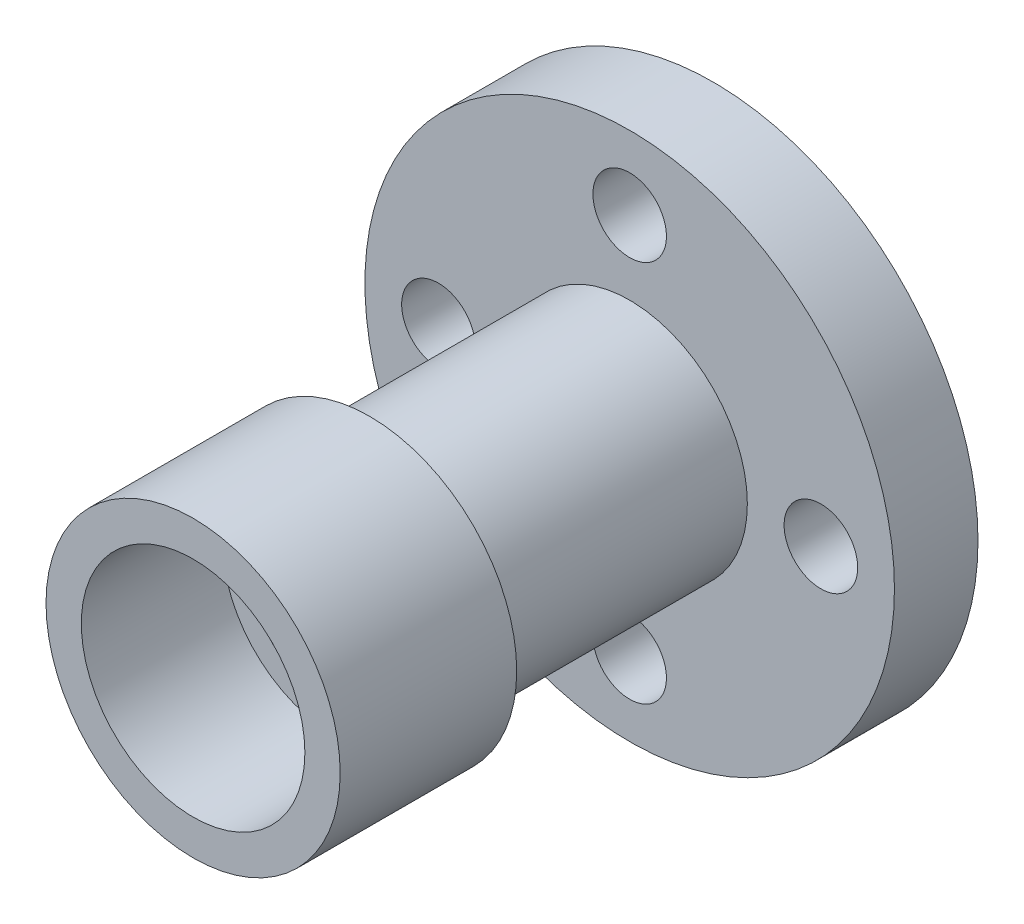
ISO-10303-21;
HEADER;
FILE_DESCRIPTION(('STEP AP214'),'2;1');
FILE_NAME('part.step','',(''),(''),'','','');
FILE_SCHEMA(('AUTOMOTIVE_DESIGN { 1 0 10303 214 1 1 1 1 }'));
ENDSEC;
DATA;
#1=APPLICATION_CONTEXT('core data for automotive mechanical design processes');
#2=APPLICATION_PROTOCOL_DEFINITION('international standard','automotive_design',2000,#1);
#3=PRODUCT_CONTEXT('',#1,'mechanical');
#4=PRODUCT('Part','Part','',(#3));
#5=PRODUCT_RELATED_PRODUCT_CATEGORY('part','',(#4));
#6=PRODUCT_DEFINITION_FORMATION('','',#4);
#7=PRODUCT_DEFINITION_CONTEXT('part definition',#1,'design');
#8=PRODUCT_DEFINITION('design','',#6,#7);
#9=PRODUCT_DEFINITION_SHAPE('','',#8);
#10=(LENGTH_UNIT() NAMED_UNIT(*) SI_UNIT(.MILLI.,.METRE.));
#11=(NAMED_UNIT(*) PLANE_ANGLE_UNIT() SI_UNIT($,.RADIAN.));
#12=(NAMED_UNIT(*) SI_UNIT($,.STERADIAN.) SOLID_ANGLE_UNIT());
#13=UNCERTAINTY_MEASURE_WITH_UNIT(LENGTH_MEASURE(1.E-05),#10,'distance_accuracy_value','');
#14=(GEOMETRIC_REPRESENTATION_CONTEXT(3) GLOBAL_UNCERTAINTY_ASSIGNED_CONTEXT((#13)) GLOBAL_UNIT_ASSIGNED_CONTEXT((#10,
#11,#12)) REPRESENTATION_CONTEXT('',''));
#15=CARTESIAN_POINT('',(0.,0.,0.));
#16=DIRECTION('',(0.,0.,1.));
#17=DIRECTION('',(1.,0.,0.));
#18=AXIS2_PLACEMENT_3D('',#15,#16,#17);
#19=CARTESIAN_POINT('',(0.,0.,64.4));
#20=DIRECTION('',(0.,0.,1.));
#21=DIRECTION('',(1.,0.,0.));
#22=AXIS2_PLACEMENT_3D('',#19,#20,#21);
#23=PLANE('',#22);
#24=CARTESIAN_POINT('',(0.,0.,64.4));
#25=DIRECTION('',(0.,0.,1.));
#26=DIRECTION('',(1.,0.,0.));
#27=AXIS2_PLACEMENT_3D('',#24,#25,#26);
#28=CIRCLE('',#27,15.);
#29=CARTESIAN_POINT('',(15.,0.,64.4));
#30=VERTEX_POINT('',#29);
#31=EDGE_CURVE('E82',#30,#30,#28,.T.);
#32=ORIENTED_EDGE('',*,*,#31,.F.);
#33=EDGE_LOOP('',(#32));
#34=FACE_BOUND('',#33,.T.);
#35=CARTESIAN_POINT('',(0.,0.,64.4));
#36=DIRECTION('',(0.,0.,1.));
#37=DIRECTION('',(1.,0.,0.));
#38=AXIS2_PLACEMENT_3D('',#35,#36,#37);
#39=CIRCLE('',#38,19.);
#40=CARTESIAN_POINT('',(19.,0.,64.4));
#41=VERTEX_POINT('',#40);
#42=EDGE_CURVE('E86',#41,#41,#39,.T.);
#43=ORIENTED_EDGE('',*,*,#42,.T.);
#44=EDGE_LOOP('',(#43));
#45=FACE_BOUND('',#44,.T.);
#46=ADVANCED_FACE('F51',(#34,#45),#23,.T.);
#47=CARTESIAN_POINT('',(0.,0.,14.2));
#48=DIRECTION('',(0.,0.,1.));
#49=DIRECTION('',(1.,0.,0.));
#50=AXIS2_PLACEMENT_3D('',#47,#48,#49);
#51=PLANE('',#50);
#52=CARTESIAN_POINT('',(32.5,0.,14.2));
#53=DIRECTION('',(0.,0.,1.));
#54=DIRECTION('',(1.,0.,0.));
#55=AXIS2_PLACEMENT_3D('',#52,#53,#54);
#56=CIRCLE('',#55,6.25);
#57=CARTESIAN_POINT('',(38.75,0.,14.2));
#58=VERTEX_POINT('',#57);
#59=EDGE_CURVE('E103',#58,#58,#56,.F.);
#60=ORIENTED_EDGE('',*,*,#59,.T.);
#61=EDGE_LOOP('',(#60));
#62=FACE_BOUND('',#61,.T.);
#63=CARTESIAN_POINT('',(-32.5,0.,14.2));
#64=DIRECTION('',(0.,0.,1.));
#65=DIRECTION('',(1.,0.,0.));
#66=AXIS2_PLACEMENT_3D('',#63,#64,#65);
#67=CIRCLE('',#66,6.25);
#68=CARTESIAN_POINT('',(-26.25,0.,14.2));
#69=VERTEX_POINT('',#68);
#70=EDGE_CURVE('E107',#69,#69,#67,.F.);
#71=ORIENTED_EDGE('',*,*,#70,.T.);
#72=EDGE_LOOP('',(#71));
#73=FACE_BOUND('',#72,.T.);
#74=CARTESIAN_POINT('',(0.,-32.5,14.2));
#75=DIRECTION('',(0.,0.,1.));
#76=DIRECTION('',(1.,0.,0.));
#77=AXIS2_PLACEMENT_3D('',#74,#75,#76);
#78=CIRCLE('',#77,6.25);
#79=CARTESIAN_POINT('',(6.25000000000001,-32.5,14.2));
#80=VERTEX_POINT('',#79);
#81=EDGE_CURVE('E93',#80,#80,#78,.F.);
#82=ORIENTED_EDGE('',*,*,#81,.T.);
#83=EDGE_LOOP('',(#82));
#84=FACE_BOUND('',#83,.T.);
#85=CARTESIAN_POINT('',(0.,32.5,14.2));
#86=DIRECTION('',(0.,0.,1.));
#87=DIRECTION('',(1.,0.,0.));
#88=AXIS2_PLACEMENT_3D('',#85,#86,#87);
#89=CIRCLE('',#88,6.25);
#90=CARTESIAN_POINT('',(6.25,32.5,14.2));
#91=VERTEX_POINT('',#90);
#92=EDGE_CURVE('E96',#91,#91,#89,.F.);
#93=ORIENTED_EDGE('',*,*,#92,.T.);
#94=EDGE_LOOP('',(#93));
#95=FACE_BOUND('',#94,.T.);
#96=CARTESIAN_POINT('',(0.,0.,14.2));
#97=DIRECTION('',(0.,0.,1.));
#98=DIRECTION('',(1.,0.,0.));
#99=AXIS2_PLACEMENT_3D('',#96,#97,#98);
#100=CIRCLE('',#99,45.);
#101=CARTESIAN_POINT('',(45.,0.,14.2));
#102=VERTEX_POINT('',#101);
#103=EDGE_CURVE('E61',#102,#102,#100,.T.);
#104=ORIENTED_EDGE('',*,*,#103,.T.);
#105=EDGE_LOOP('',(#104));
#106=FACE_BOUND('',#105,.T.);
#107=CARTESIAN_POINT('',(0.,0.,14.2));
#108=DIRECTION('',(0.,0.,1.));
#109=DIRECTION('',(1.,0.,0.));
#110=AXIS2_PLACEMENT_3D('',#107,#108,#109);
#111=CIRCLE('',#110,20.);
#112=CARTESIAN_POINT('',(20.,0.,14.2));
#113=VERTEX_POINT('',#112);
#114=EDGE_CURVE('E71',#113,#113,#111,.T.);
#115=ORIENTED_EDGE('',*,*,#114,.F.);
#116=EDGE_LOOP('',(#115));
#117=FACE_BOUND('',#116,.T.);
#118=ADVANCED_FACE('F132',(#62,#73,#84,#95,#106,#117),#51,.T.);
#119=CARTESIAN_POINT('',(0.,0.,0.));
#120=DIRECTION('',(0.,0.,1.));
#121=DIRECTION('',(1.,0.,0.));
#122=AXIS2_PLACEMENT_3D('',#119,#120,#121);
#123=PLANE('',#122);
#124=CARTESIAN_POINT('',(32.5,0.,0.));
#125=DIRECTION('',(0.,0.,1.));
#126=DIRECTION('',(1.,0.,0.));
#127=AXIS2_PLACEMENT_3D('',#124,#125,#126);
#128=CIRCLE('',#127,6.25);
#129=CARTESIAN_POINT('',(38.75,0.,0.));
#130=VERTEX_POINT('',#129);
#131=EDGE_CURVE('E112',#130,#130,#128,.T.);
#132=ORIENTED_EDGE('',*,*,#131,.T.);
#133=EDGE_LOOP('',(#132));
#134=FACE_BOUND('',#133,.T.);
#135=CARTESIAN_POINT('',(-32.5,0.,0.));
#136=DIRECTION('',(0.,0.,1.));
#137=DIRECTION('',(1.,0.,0.));
#138=AXIS2_PLACEMENT_3D('',#135,#136,#137);
#139=CIRCLE('',#138,6.25);
#140=CARTESIAN_POINT('',(-26.25,0.,0.));
#141=VERTEX_POINT('',#140);
#142=EDGE_CURVE('E115',#141,#141,#139,.T.);
#143=ORIENTED_EDGE('',*,*,#142,.T.);
#144=EDGE_LOOP('',(#143));
#145=FACE_BOUND('',#144,.T.);
#146=CARTESIAN_POINT('',(0.,-32.5,0.));
#147=DIRECTION('',(0.,0.,1.));
#148=DIRECTION('',(1.,0.,0.));
#149=AXIS2_PLACEMENT_3D('',#146,#147,#148);
#150=CIRCLE('',#149,6.25);
#151=CARTESIAN_POINT('',(6.25000000000001,-32.5,0.));
#152=VERTEX_POINT('',#151);
#153=EDGE_CURVE('E97',#152,#152,#150,.T.);
#154=ORIENTED_EDGE('',*,*,#153,.T.);
#155=EDGE_LOOP('',(#154));
#156=FACE_BOUND('',#155,.T.);
#157=CARTESIAN_POINT('',(0.,32.5,0.));
#158=DIRECTION('',(0.,0.,1.));
#159=DIRECTION('',(1.,0.,0.));
#160=AXIS2_PLACEMENT_3D('',#157,#158,#159);
#161=CIRCLE('',#160,6.25);
#162=CARTESIAN_POINT('',(6.25,32.5,0.));
#163=VERTEX_POINT('',#162);
#164=EDGE_CURVE('E99',#163,#163,#161,.T.);
#165=ORIENTED_EDGE('',*,*,#164,.T.);
#166=EDGE_LOOP('',(#165));
#167=FACE_BOUND('',#166,.T.);
#168=CARTESIAN_POINT('',(0.,0.,0.));
#169=DIRECTION('',(0.,0.,1.));
#170=DIRECTION('',(1.,0.,0.));
#171=AXIS2_PLACEMENT_3D('',#168,#169,#170);
#172=CIRCLE('',#171,18.5);
#173=CARTESIAN_POINT('',(18.5,0.,0.));
#174=VERTEX_POINT('',#173);
#175=EDGE_CURVE('E56',#174,#174,#172,.T.);
#176=ORIENTED_EDGE('',*,*,#175,.T.);
#177=EDGE_LOOP('',(#176));
#178=FACE_BOUND('',#177,.T.);
#179=CARTESIAN_POINT('',(0.,0.,0.));
#180=DIRECTION('',(0.,0.,1.));
#181=DIRECTION('',(1.,0.,0.));
#182=AXIS2_PLACEMENT_3D('',#179,#180,#181);
#183=CIRCLE('',#182,45.);
#184=CARTESIAN_POINT('',(45.,0.,0.));
#185=VERTEX_POINT('',#184);
#186=EDGE_CURVE('E69',#185,#185,#183,.T.);
#187=ORIENTED_EDGE('',*,*,#186,.F.);
#188=EDGE_LOOP('',(#187));
#189=FACE_BOUND('',#188,.T.);
#190=ADVANCED_FACE('F116',(#134,#145,#156,#167,#178,#189),#123,.F.);
#191=CARTESIAN_POINT('',(0.,0.,14.2));
#192=DIRECTION('',(0.,0.,-1.));
#193=DIRECTION('',(-1.,0.,0.));
#194=AXIS2_PLACEMENT_3D('',#191,#192,#193);
#195=CYLINDRICAL_SURFACE('',#194,45.);
#196=ORIENTED_EDGE('',*,*,#103,.F.);
#197=EDGE_LOOP('',(#196));
#198=FACE_BOUND('',#197,.T.);
#199=ORIENTED_EDGE('',*,*,#186,.T.);
#200=EDGE_LOOP('',(#199));
#201=FACE_BOUND('',#200,.T.);
#202=ADVANCED_FACE('F165',(#198,#201),#195,.T.);
#203=CARTESIAN_POINT('',(0.,0.,14.2));
#204=DIRECTION('',(0.,0.,-1.));
#205=DIRECTION('',(-1.,0.,0.));
#206=AXIS2_PLACEMENT_3D('',#203,#204,#205);
#207=CYLINDRICAL_SURFACE('',#206,15.);
#208=CARTESIAN_POINT('',(0.,0.,3.));
#209=DIRECTION('',(0.,0.,1.));
#210=DIRECTION('',(1.,0.,0.));
#211=AXIS2_PLACEMENT_3D('',#208,#209,#210);
#212=CIRCLE('',#211,15.);
#213=CARTESIAN_POINT('',(15.,0.,3.));
#214=VERTEX_POINT('',#213);
#215=EDGE_CURVE('E12',#214,#214,#212,.F.);
#216=ORIENTED_EDGE('',*,*,#215,.T.);
#217=EDGE_LOOP('',(#216));
#218=FACE_BOUND('',#217,.T.);
#219=ORIENTED_EDGE('',*,*,#31,.T.);
#220=EDGE_LOOP('',(#219));
#221=FACE_BOUND('',#220,.T.);
#222=ADVANCED_FACE('F157',(#218,#221),#207,.F.);
#223=CARTESIAN_POINT('',(0.,0.,58.4));
#224=DIRECTION('',(0.,0.,-1.));
#225=DIRECTION('',(-1.,0.,0.));
#226=AXIS2_PLACEMENT_3D('',#223,#224,#225);
#227=CYLINDRICAL_SURFACE('',#226,20.);
#228=CARTESIAN_POINT('',(0.,0.,58.4));
#229=DIRECTION('',(0.,0.,1.));
#230=DIRECTION('',(1.,0.,0.));
#231=AXIS2_PLACEMENT_3D('',#228,#229,#230);
#232=CIRCLE('',#231,20.);
#233=CARTESIAN_POINT('',(20.,0.,58.4));
#234=VERTEX_POINT('',#233);
#235=EDGE_CURVE('E72',#234,#234,#232,.T.);
#236=ORIENTED_EDGE('',*,*,#235,.F.);
#237=EDGE_LOOP('',(#236));
#238=FACE_BOUND('',#237,.T.);
#239=ORIENTED_EDGE('',*,*,#114,.T.);
#240=EDGE_LOOP('',(#239));
#241=FACE_BOUND('',#240,.T.);
#242=ADVANCED_FACE('F153',(#238,#241),#227,.T.);
#243=CARTESIAN_POINT('',(0.,0.,58.4));
#244=DIRECTION('',(0.,0.,1.));
#245=DIRECTION('',(1.,0.,0.));
#246=AXIS2_PLACEMENT_3D('',#243,#244,#245);
#247=PLANE('',#246);
#248=ORIENTED_EDGE('',*,*,#235,.T.);
#249=EDGE_LOOP('',(#248));
#250=FACE_BOUND('',#249,.T.);
#251=CARTESIAN_POINT('',(0.,0.,58.4));
#252=DIRECTION('',(0.,0.,1.));
#253=DIRECTION('',(1.,0.,0.));
#254=AXIS2_PLACEMENT_3D('',#251,#252,#253);
#255=CIRCLE('',#254,25.);
#256=CARTESIAN_POINT('',(25.,0.,58.4));
#257=VERTEX_POINT('',#256);
#258=EDGE_CURVE('E78',#257,#257,#255,.T.);
#259=ORIENTED_EDGE('',*,*,#258,.F.);
#260=EDGE_LOOP('',(#259));
#261=FACE_BOUND('',#260,.T.);
#262=ADVANCED_FACE('F147',(#250,#261),#247,.F.);
#263=CARTESIAN_POINT('',(0.,0.,64.4));
#264=DIRECTION('',(0.,0.,-1.));
#265=DIRECTION('',(-1.,0.,0.));
#266=AXIS2_PLACEMENT_3D('',#263,#264,#265);
#267=CYLINDRICAL_SURFACE('',#266,25.);
#268=ORIENTED_EDGE('',*,*,#258,.T.);
#269=EDGE_LOOP('',(#268));
#270=FACE_BOUND('',#269,.T.);
#271=CARTESIAN_POINT('',(0.,0.,88.4));
#272=DIRECTION('',(0.,0.,1.));
#273=DIRECTION('',(1.,0.,0.));
#274=AXIS2_PLACEMENT_3D('',#271,#272,#273);
#275=CIRCLE('',#274,25.);
#276=CARTESIAN_POINT('',(25.,0.,88.4));
#277=VERTEX_POINT('',#276);
#278=EDGE_CURVE('E81',#277,#277,#275,.T.);
#279=ORIENTED_EDGE('',*,*,#278,.F.);
#280=EDGE_LOOP('',(#279));
#281=FACE_BOUND('',#280,.T.);
#282=ADVANCED_FACE('F155',(#270,#281),#267,.T.);
#283=CARTESIAN_POINT('',(0.,0.,88.4));
#284=DIRECTION('',(0.,0.,1.));
#285=DIRECTION('',(1.,0.,0.));
#286=AXIS2_PLACEMENT_3D('',#283,#284,#285);
#287=PLANE('',#286);
#288=ORIENTED_EDGE('',*,*,#278,.T.);
#289=EDGE_LOOP('',(#288));
#290=FACE_BOUND('',#289,.T.);
#291=CARTESIAN_POINT('',(0.,0.,88.4));
#292=DIRECTION('',(0.,0.,1.));
#293=DIRECTION('',(1.,0.,0.));
#294=AXIS2_PLACEMENT_3D('',#291,#292,#293);
#295=CIRCLE('',#294,19.);
#296=CARTESIAN_POINT('',(19.,0.,88.4));
#297=VERTEX_POINT('',#296);
#298=EDGE_CURVE('E87',#297,#297,#295,.T.);
#299=ORIENTED_EDGE('',*,*,#298,.F.);
#300=EDGE_LOOP('',(#299));
#301=FACE_BOUND('',#300,.T.);
#302=ADVANCED_FACE('F146',(#290,#301),#287,.T.);
#303=CARTESIAN_POINT('',(0.,0.,88.4));
#304=DIRECTION('',(0.,0.,-1.));
#305=DIRECTION('',(-1.,0.,0.));
#306=AXIS2_PLACEMENT_3D('',#303,#304,#305);
#307=CYLINDRICAL_SURFACE('',#306,19.);
#308=ORIENTED_EDGE('',*,*,#298,.T.);
#309=EDGE_LOOP('',(#308));
#310=FACE_BOUND('',#309,.T.);
#311=ORIENTED_EDGE('',*,*,#42,.F.);
#312=EDGE_LOOP('',(#311));
#313=FACE_BOUND('',#312,.T.);
#314=ADVANCED_FACE('F212',(#310,#313),#307,.F.);
#315=CARTESIAN_POINT('',(0.,0.,0.));
#316=DIRECTION('',(0.,0.,-1.));
#317=DIRECTION('',(-1.,0.,0.));
#318=AXIS2_PLACEMENT_3D('',#315,#316,#317);
#319=CONICAL_SURFACE('',#318,18.5,0.862170054667226);
#320=ORIENTED_EDGE('',*,*,#215,.F.);
#321=EDGE_LOOP('',(#320));
#322=FACE_BOUND('',#321,.T.);
#323=ORIENTED_EDGE('',*,*,#175,.F.);
#324=EDGE_LOOP('',(#323));
#325=FACE_BOUND('',#324,.T.);
#326=ADVANCED_FACE('F53',(#322,#325),#319,.F.);
#327=CARTESIAN_POINT('',(0.,32.5,24.));
#328=DIRECTION('',(0.,0.,-1.));
#329=DIRECTION('',(-1.,0.,0.));
#330=AXIS2_PLACEMENT_3D('',#327,#328,#329);
#331=CYLINDRICAL_SURFACE('',#330,6.25);
#332=ORIENTED_EDGE('',*,*,#92,.F.);
#333=EDGE_LOOP('',(#332));
#334=FACE_BOUND('',#333,.T.);
#335=ORIENTED_EDGE('',*,*,#164,.F.);
#336=EDGE_LOOP('',(#335));
#337=FACE_BOUND('',#336,.T.);
#338=ADVANCED_FACE('F227',(#334,#337),#331,.F.);
#339=CARTESIAN_POINT('',(0.,-32.5,24.));
#340=DIRECTION('',(0.,0.,-1.));
#341=DIRECTION('',(-1.,0.,0.));
#342=AXIS2_PLACEMENT_3D('',#339,#340,#341);
#343=CYLINDRICAL_SURFACE('',#342,6.25);
#344=ORIENTED_EDGE('',*,*,#81,.F.);
#345=EDGE_LOOP('',(#344));
#346=FACE_BOUND('',#345,.T.);
#347=ORIENTED_EDGE('',*,*,#153,.F.);
#348=EDGE_LOOP('',(#347));
#349=FACE_BOUND('',#348,.T.);
#350=ADVANCED_FACE('F129',(#346,#349),#343,.F.);
#351=CARTESIAN_POINT('',(-32.5,0.,24.));
#352=DIRECTION('',(0.,0.,-1.));
#353=DIRECTION('',(-1.,0.,0.));
#354=AXIS2_PLACEMENT_3D('',#351,#352,#353);
#355=CYLINDRICAL_SURFACE('',#354,6.25);
#356=ORIENTED_EDGE('',*,*,#70,.F.);
#357=EDGE_LOOP('',(#356));
#358=FACE_BOUND('',#357,.T.);
#359=ORIENTED_EDGE('',*,*,#142,.F.);
#360=EDGE_LOOP('',(#359));
#361=FACE_BOUND('',#360,.T.);
#362=ADVANCED_FACE('F125',(#358,#361),#355,.F.);
#363=CARTESIAN_POINT('',(32.5,0.,24.));
#364=DIRECTION('',(0.,0.,-1.));
#365=DIRECTION('',(-1.,0.,0.));
#366=AXIS2_PLACEMENT_3D('',#363,#364,#365);
#367=CYLINDRICAL_SURFACE('',#366,6.25);
#368=ORIENTED_EDGE('',*,*,#59,.F.);
#369=EDGE_LOOP('',(#368));
#370=FACE_BOUND('',#369,.T.);
#371=ORIENTED_EDGE('',*,*,#131,.F.);
#372=EDGE_LOOP('',(#371));
#373=FACE_BOUND('',#372,.T.);
#374=ADVANCED_FACE('F122',(#370,#373),#367,.F.);
#375=CLOSED_SHELL('',(#46,#118,#190,#202,#222,#242,#262,#282,#302,#314,#326,#338,#350,#362,#374));
#376=MANIFOLD_SOLID_BREP('B2',#375);
#377=ADVANCED_BREP_SHAPE_REPRESENTATION('',(#18,#376),#14);
#378=SHAPE_DEFINITION_REPRESENTATION(#9,#377);
ENDSEC;
END-ISO-10303-21;
